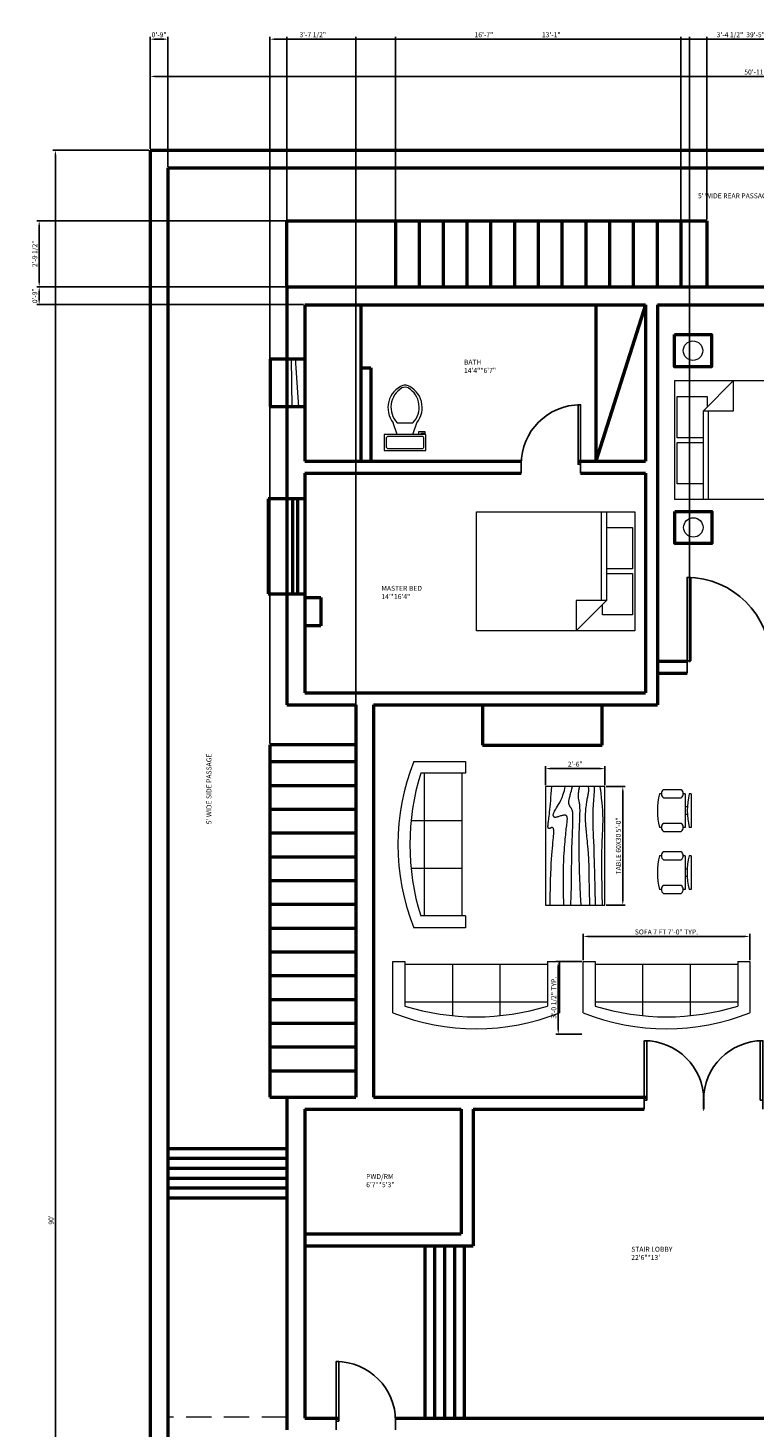
# Model space of a CAD drawing. Units: inches. Extents: x 5312 to 23584, y 2846 to 7447.
# Tile 10 of 12: x 11386 to 11753, y 3367 to 4074. Entities that reach past the tile are written whole.
import ezdxf

# ---------------------------------------------------------------- set-up
doc = ezdxf.new("R2010")
doc.units = ezdxf.units.IN
doc.linetypes.add('DASHED', pattern=[19.05, 12.7, -6.35])
for name, color, linetype, lineweight in [('A-ANNO-DIMS', 2, 'Continuous', 18), ('A-ANNO-TEXT', 3, 'Continuous', 18), ('A-AREA-IDEN', 7, 'Continuous', 18), ('A-DOOR', 4, 'Continuous', 25), ('A-FLOR-FIXT', 9, 'Continuous', 18), ('A-FLOR-OVHD', 8, 'DASHED', 18), ('A-FURN', 8, 'Continuous', 18), ('A-WALL', 7, 'Continuous', 50)]:
    doc.layers.add(name, color=color, linetype=linetype, lineweight=lineweight)
doc.styles.get("Standard").update_dxf_attribs({"font": 'arial.ttf'})
doc.dimstyles.new('ISO-25', dxfattribs={"dimtxt": 2.5, "dimasz": 2.5, "dimexe": 1.25, "dimexo": 0.625, "dimtad": 1, "dimlunit": 3, "dimtxsty": 'Standard', "dimcen": 2.5, "dimadec": 0, "dimazin": 0, "dimtfac": 1, "dimtmove": 0, "dimatfit": 3, "dimfxl": 1, "dimarcsym": 0})

# ---------------------------------------------------------------- blocks, each defined once
blk = doc.blocks.new('*U2')
for p, q in [((0, 0), (0, -6)), ((40, 0), (40, -6))]:
    blk.add_line(p, q)
blk.add_lwpolyline([(0, 0), (0, 40), (1.75, 40), (1.75, 0)], close=True)
blk.add_arc((0, 0), 40, 0, 90)
blk = doc.blocks.new('Toilet - top')
for p, q in [((9.5, -6), (9.5, -2)), ((-10, -8.5), (-8, -8.5)), ((-10, -9.5), (-10, -8.5)), ((-7, -9.5), (-10, -9.5)), ((-8, -8.5), (-8, -8)), ((-7, -8), (-7, -9.5)), ((-4, -8), (-6, -14)), ((4, -14), (-4, -14)), ((4, -8), (6, -14))]:
    blk.add_line(p, q)
blk.add_lwpolyline([(10.5, -8), (10.5, 0), (-10.5, 0), (-10.5, -8)], close=True)
for points in [[(-9.5, -2), (-9.5, -6)], [(8.5, -1), (-8.5, -1)], [(-8.5, -7), (8.5, -7)]]:
    blk.add_lwpolyline(points)
for centre, radius, start, end in [((-8.62, -1.88), 0.884, 81.8699, 188.1301), ((-8.62, -6.12), 0.884, 171.8699, 278.1301), ((8.62, -1.88), 0.884, 351.8699, 98.1301), ((8.62, -6.12), 0.884, 261.8699, 8.1301), ((3.52, -21.58), 12.17, 141.46911, 247.97143), ((4.2, -21.82), 11.33, 136.36773, 238.94682), ((-3.52, -21.58), 12.17, 292.02843, 38.53071), ((-4.2, -21.82), 11.33, 301.05301, 43.63209), ((0, -27.88), 4, 245.73182, 294.26817), ((0, -29), 4, 254.86053, 285.13947)]:
    blk.add_arc(centre, radius, start, end)
blk = doc.blocks.new('Bed - Queen')
for p, q in [((0, -80.00003), (0, 0)), ((0, 0), (59.99999, 0)), ((59.99999, 0), (59.99999, -80.00003)), ((7.99999, -1.2), (28.79998, -1.2)), ((7.99999, -14.4), (7.99999, -1.2)), ((28.79998, -1.2), (28.79998, -14.4)), ((31.19999, -1.2), (51.99999, -1.2)), ((31.19999, -14.4), (31.19999, -1.2)), ((51.99999, -1.2), (51.99999, -16.4)), ((0, -14.4), (44.8, -14.4)), ((44.8, -16.8), (0, -16.8)), ((59.99999, -29.6), (44.8, -14.4)), ((44.8, -14.4), (44.8, -29.6)), ((51.99999, -16.4), (46.79936, -16.4)), ((44.8, -29.6), (59.99999, -29.6)), ((59.99999, -80.00003), (0, -80.00003))]:
    blk.add_line(p, q)
blk = doc.blocks.new('Sofa - Roundback 7 ft.')
for p, q in [((-12.00002, -32.4421), (-12.00003, -6.5971)), ((11.99997, -32.4421), (11.99998, -6.5971)), ((-36.000027, -34), (-36.000027, -11.4696)), ((-35.999844, -13.3819), (35.9998, -13.3819)), ((35.99998, -34), (35.99998, -11.4696)), ((-36.000027, -32.4421), (35.99998, -32.4421))]:
    blk.add_line(p, q)
for points in [[(-36.000027, -34), (-42.000027, -34), (-42.000027, -8)], [(41.99998, -8), (41.99998, -34), (35.99998, -34)]]:
    blk.add_lwpolyline(points)
for centre, radius, start, end in [((0, -114.25), 114.25, 68.43141, 111.5686), ((-0.00001, -127.1968), 121.1968, 72.72033, 107.2797)]:
    blk.add_arc(centre, radius, start, end)
blk = doc.blocks.new('Table - Rectangular Woodgrain 60 x 30 in.')
for p, q in [((0, 0), (0, -30)), ((60, 0), (0, 0)), ((60, -30), (60, 0)), ((0, -30), (60, -30))]:
    blk.add_line(p, q)
for points in [[(0, -2.4), (4.8155, -2.418), (9.0302, -2.4688), (12.709, -2.5477), (15.9167, -2.65), (18.7181, -2.7711), (21.1781, -2.9063), (23.3616, -3.0508), (25.3333, -3.2), (27.1477, -3.3495), (28.8172, -3.4958), (30.3437, -3.636), (31.7291, -3.7667), (32.9756, -3.8849), (34.0849, -3.9875), (35.059, -4.0714), (35.9, -4.1334), (36.6114, -4.1711), (37.2041, -4.1854), (37.6906, -4.1779), (38.0833, -4.15), (38.3948, -4.1034), (38.6375, -4.0396), (38.8239, -3.9602), (38.9666, -3.8667), (39.0764, -3.7608), (39.1573, -3.6448), (39.2116, -3.521), (39.2416, -3.3917), (39.2498, -3.2593), (39.2385, -3.1261), (39.21, -2.9944), (39.1666, -2.8667), (39.111, -2.7447), (39.0468, -2.6281), (38.978, -2.5163), (38.9083, -2.4083), (38.8418, -2.3035), (38.7823, -2.201), (38.7337, -2.1001), (38.7, -2), (38.6844, -1.9003), (38.6875, -1.8021), (38.7094, -1.707), (38.75, -1.6167), (38.8094, -1.5326), (38.8875, -1.4563), (38.9844, -1.3893), (39.1, -1.3333), (39.2351, -1.2896), (39.3937, -1.2583), (39.5804, -1.2396), (39.8, -1.2333), (40.057, -1.2396), (40.3562, -1.2583), (40.7023, -1.2896), (41.1, -1.3333), (41.5547, -1.3895), (42.0755, -1.4573), (42.6721, -1.5361), (43.3542, -1.625), (44.1316, -1.7233), (45.014, -1.8302), (46.0114, -1.9449), (47.1333, -2.0667), (48.3862, -2.1947), (49.7625, -2.3281), (51.2513, -2.4663), (52.8416, -2.6083), (54.5226, -2.7535), (56.2833, -2.9011), (58.1127, -3.0501), (60, -3.2)], [(0, -9.2), (6.5759, -9.0858), (11.9385, -9.0365), (16.2527, -9.0418), (19.6833, -9.0917), (22.3952, -9.1759), (24.5531, -9.2844), (26.322, -9.4069), (27.8666, -9.5333), (29.3241, -9.6553), (30.7203, -9.7719), (32.0532, -9.8837), (33.3208, -9.9917), (34.5213, -10.0965), (35.6526, -10.199), (36.7128, -10.2999), (37.7, -10.4), (38.6129, -10.4996), (39.4531, -10.5969), (40.223, -10.6895), (40.925, -10.775), (41.5613, -10.8512), (42.1344, -10.9156), (42.6465, -10.966), (43.1, -11), (43.4976, -11.0158), (43.8437, -11.0136), (44.143, -10.9942), (44.4, -10.9583), (44.6195, -10.9069), (44.8062, -10.8406), (44.9648, -10.7603), (45.1, -10.6667), (45.2155, -10.5598), (45.3114, -10.4365), (45.3871, -10.2929), (45.4416, -10.125), (45.4743, -9.929), (45.4844, -9.7011), (45.4709, -9.4371), (45.4333, -9.1333), (45.3716, -8.7883), (45.2896, -8.4104), (45.1919, -8.0107), (45.0833, -7.6), (44.9685, -7.1893), (44.8521, -6.7896), (44.7388, -6.4117), (44.6333, -6.0667), (44.54, -5.7628), (44.4614, -5.4979), (44.4001, -5.2675), (44.3583, -5.0667), (44.3384, -4.8909), (44.3427, -4.7354), (44.3736, -4.5956), (44.4333, -4.4667), (44.5236, -4.3453), (44.6427, -4.2333), (44.7884, -4.1339), (44.9583, -4.05), (45.1501, -3.9849), (45.3614, -3.9417), (45.59, -3.9234), (45.8333, -3.9333), (46.0915, -3.9749), (46.3734, -4.0531), (46.6906, -4.1736), (47.0542, -4.3417), (47.4756, -4.5629), (47.9661, -4.8427), (48.5372, -5.1866), (49.2, -5.6), (49.9676, -6.0844), (50.8594, -6.625), (51.8965, -7.2031), (53.1, -7.8), (54.491, -8.3969), (56.0906, -8.975), (57.9199, -9.5156), (60, -10)], [(0, -12.8), (5.1847, -12.9322), (9.6213, -13.0323), (13.3963, -13.1059), (16.5958, -13.1583), (19.3063, -13.1952), (21.614, -13.2219), (23.6054, -13.2439), (25.3666, -13.2667), (26.9728, -13.2947), (28.4531, -13.3281), (29.8256, -13.3663), (31.1083, -13.4083), (32.3191, -13.4535), (33.476, -13.501), (34.597, -13.5501), (35.7, -13.6), (36.7984, -13.6497), (37.8875, -13.6979), (38.9578, -13.743), (40, -13.7833), (41.0047, -13.8174), (41.9625, -13.8438), (42.864, -13.8607), (43.7, -13.8667), (44.4631, -13.8604), (45.1552, -13.8417), (45.7801, -13.8104), (46.3416, -13.7667), (46.8439, -13.7104), (47.2906, -13.6417), (47.6858, -13.5604), (48.0333, -13.4667), (48.3375, -13.3608), (48.6042, -13.2448), (48.8396, -13.121), (49.05, -12.9917), (49.2417, -12.8593), (49.4208, -12.7261), (49.5937, -12.5944), (49.7667, -12.4667), (49.9452, -12.3451), (50.1323, -12.2313), (50.3303, -12.1268), (50.5416, -12.0333), (50.7686, -11.9524), (51.0135, -11.8854), (51.2788, -11.8341), (51.5666, -11.8), (51.8785, -11.7843), (52.2116, -11.7865), (52.562, -11.8059), (52.926, -11.8417), (53.2998, -11.8931), (53.6795, -11.9594), (54.0614, -12.0397), (54.4416, -12.1333), (54.8223, -12.2401), (55.2293, -12.3625), (55.6942, -12.5037), (56.2489, -12.6667), (56.9251, -12.8547), (57.7545, -13.0708), (58.7689, -13.3182), (60, -13.6)], [(0, -18), (5.124, -17.7273), (9.6609, -17.5057), (13.6705, -17.3303), (17.2125, -17.1958), (20.3467, -17.0973), (23.1328, -17.0297), (25.6307, -16.9878), (27.9, -16.9667), (29.9928, -16.9617), (31.9302, -16.9703), (33.7254, -16.9907), (35.3917, -17.0208), (36.9423, -17.0588), (38.3906, -17.1026), (39.7499, -17.1503), (41.0333, -17.2), (42.2519, -17.2496), (43.4073, -17.2969), (44.4986, -17.3395), (45.525, -17.375), (46.4858, -17.4012), (47.3802, -17.4156), (48.2074, -17.416), (48.9667, -17.4), (49.6583, -17.3662), (50.2872, -17.3167), (50.8595, -17.2547), (51.3812, -17.1833), (51.8584, -17.1057), (52.2971, -17.025), (52.7034, -16.9443), (53.0833, -16.8667), (53.443, -16.7951), (53.789, -16.7313), (54.128, -16.6768), (54.4666, -16.6334), (54.8115, -16.6024), (55.1693, -16.5854), (55.5465, -16.5841), (55.95, -16.6), (56.3828, -16.6337), (56.8346, -16.6823), (57.2915, -16.7418), (57.7396, -16.8084), (58.165, -16.878), (58.5539, -16.9469), (58.8924, -17.0111), (59.1666, -17.0667), (59.3679, -17.1107), (59.5078, -17.1438), (59.6032, -17.1675), (59.6708, -17.1833), (59.7275, -17.193), (59.7901, -17.1979), (59.8753, -17.1998), (60, -17.2)], [(0, -22.4), (8.0098, -22.2501), (14.4094, -22.1011), (19.4168, -21.9535), (23.25, -21.8083), (26.1269, -21.6663), (28.2656, -21.5281), (29.884, -21.3947), (31.2, -21.2667), (32.3967, -21.1448), (33.5172, -21.0292), (34.5697, -20.9198), (35.5625, -20.8167), (36.5037, -20.7198), (37.4015, -20.6292), (38.2642, -20.5448), (39.1, -20.4667), (39.9164, -20.3951), (40.7187, -20.3313), (41.5117, -20.2768), (42.3, -20.2333), (43.0883, -20.2024), (43.8812, -20.1854), (44.6836, -20.1841), (45.5, -20.2), (46.3328, -20.234), (47.1747, -20.2844), (48.0163, -20.3488), (48.8479, -20.425), (49.66, -20.5106), (50.4429, -20.6031), (51.1872, -20.7004), (51.8833, -20.8), (52.5246, -20.8999), (53.1166, -20.9995), (53.6681, -21.0983), (54.1875, -21.1958), (54.6834, -21.2919), (55.1646, -21.3859), (55.6394, -21.4777), (56.1167, -21.5667), (56.6028, -21.6515), (57.0961, -21.7266), (57.5929, -21.7852), (58.0896, -21.8208), (58.5823, -21.8268), (59.0674, -21.7964), (59.5412, -21.723), (60, -21.6)], [(0, -25.2), (8.6355, -25.0504), (15.7026, -24.9031), (21.4049, -24.7606), (25.9458, -24.625), (29.529, -24.4988), (32.3578, -24.3844), (34.6359, -24.284), (36.5667, -24.2), (38.3213, -24.1341), (39.9417, -24.0854), (41.437, -24.0523), (42.8167, -24.0333), (44.0901, -24.0268), (45.2667, -24.0313), (46.3557, -24.0451), (47.3667, -24.0667), (48.309, -24.0947), (49.1928, -24.1287), (50.0284, -24.168), (50.826, -24.2125), (51.5959, -24.2617), (52.3483, -24.3151), (53.0935, -24.3725), (53.8417, -24.4334), (54.6009, -24.497), (55.3699, -24.561), (56.1454, -24.6226), (56.9239, -24.6792), (57.7021, -24.7279), (58.4764, -24.7662), (59.2435, -24.7911), (60, -24.8)], [(0, -28.8), (5.6867, -28.6681), (10.45, -28.5698), (14.407, -28.5012), (17.675, -28.4584), (20.3711, -28.4374), (22.6125, -28.4344), (24.5164, -28.4455), (26.2, -28.4667), (27.762, -28.4947), (29.2276, -28.5281), (30.6033, -28.5663), (31.8958, -28.6084), (33.1118, -28.6535), (34.2578, -28.7011), (35.3405, -28.7501), (36.3666, -28.8), (37.3443, -28.8497), (38.288, -28.8974), (39.2137, -28.9412), (40.1375, -28.9792), (41.0753, -29.0093), (42.0432, -29.0297), (43.0572, -29.0384), (44.1333, -29.0333), (45.2936, -29.0114), (46.5843, -28.9641), (48.0579, -28.8816), (49.7666, -28.7542), (51.7629, -28.5721), (54.0989, -28.3255), (56.8272, -28.0048), (60, -27.6)]]:
    blk.add_lwpolyline(points)
blk = doc.blocks.new('Chair - Desk')
for p, q in [((-8.5, 0), (-8.5, -1)), ((-8.5, 0), (8.5, 0)), ((8.5, 0), (8.5, -1)), ((-10.5, -5), (-10.5, -14)), ((-8.5, -3), (-8.5, -4)), ((-8.5, -3), (8.5, -3)), ((-6.5, -14), (-6.5, -5)), ((-2, -3), (-2, -1.9355)), ((2, -1.9576), (2, -3)), ((6.5, -5), (6.5, -14)), ((8.5, -3), (8.5, -4)), ((10.5, -14), (10.5, -5)), ((-8.5, -15), (-8.5, -16)), ((8.5, -15), (8.5, -16))]:
    blk.add_line(p, q)
for centre, radius, start, end in [((-8.5, -6.5), 2.5, 36.8699, 143.1301), ((0, 34.625), 36.625, 256.5803, 283.4197), ((8.5, -6.5), 2.5, 36.8699, 143.1301), ((-8.5, -12.5), 2.5, 216.8699, 323.1301), ((8.5, -12.5), 2.5, 216.8699, 323.1301), ((0, 19.625), 36.625, 256.5803, 283.4197)]:
    blk.add_arc(centre, radius, start, end)
blk = doc.blocks.new('*D19')
at = {"layer": 'A-ANNO-DIMS', "color": 0, "lineweight": -2, "transparency": 16777216}
for p, q in [((11447.29, 4012.53), (11447.29, 4050.35)), ((11449.79, 4049.1), (12055.79, 4049.1)), ((12058.29, 4012.53), (12058.29, 4050.35))]:
    blk.add_line(p, q, dxfattribs=at)
at = {"layer": 'A-ANNO-DIMS', "color": 0, "transparency": 16777216}
for points in [[(11449.79, 4049.52), (11449.79, 4048.69), (11447.29, 4049.1)], [(12055.79, 4049.52), (12055.79, 4048.69), (12058.29, 4049.1)]]:
    blk.add_solid(points, dxfattribs=at)
at = {"layer": 'DEFPOINTS', "color": 0, "transparency": 16777216}
for p in [(12058.29, 4049.1), (11447.29, 4011.91), (12058.29, 4011.91)]:
    blk.add_point(p, dxfattribs=at)
at = {"layer": 'A-ANNO-DIMS', "color": 0, "transparency": 16777216, "insert": (11752.79, 4051.01), "char_height": 2.5, "attachment_point": 5}
blk.add_mtext('50\'-11"', dxfattribs=at)
blk = doc.blocks.new('*D20')
at = {"layer": 'A-ANNO-DIMS', "color": 0, "lineweight": -2, "transparency": 16777216}
for p, q in [((11446.67, 4011.91), (11398.24, 4011.91)), ((11399.49, 4009.41), (11399.49, 2934.41)), ((11446.67, 2931.91), (11398.24, 2931.91))]:
    blk.add_line(p, q, dxfattribs=at)
at = {"layer": 'A-ANNO-DIMS', "color": 0, "transparency": 16777216}
for points in [[(11399.07, 4009.41), (11399.9, 4009.41), (11399.49, 4011.91)], [(11399.07, 2934.41), (11399.9, 2934.41), (11399.49, 2931.91)]]:
    blk.add_solid(points, dxfattribs=at)
at = {"layer": 'DEFPOINTS', "color": 0, "transparency": 16777216}
for p in [(11447.29, 4011.91), (11399.49, 2931.91), (11447.29, 2931.91)]:
    blk.add_point(p, dxfattribs=at)
at = {"layer": 'A-ANNO-DIMS', "color": 0, "transparency": 16777216, "insert": (11397.59, 3471.91), "char_height": 2.5, "attachment_point": 5, "rotation": 90}
blk.add_mtext("90'", dxfattribs=at)
blk = doc.blocks.new('WARDROBE-HANGER')
for p, q in [((0, 3.4), (24.8, 3.4)), ((0, 1.32), (24.99, 0))]:
    blk.add_line(p, q)
blk = doc.blocks.new('*D27')
at = {"layer": 'A-ANNO-DIMS', "color": 0, "lineweight": -2, "transparency": 16777216}
for p, q in [((11665.83, 3603.06), (11665.83, 3616.28)), ((11747.33, 3615.03), (11668.33, 3615.03)), ((11749.83, 3603.06), (11749.83, 3616.28))]:
    blk.add_line(p, q, dxfattribs=at)
at = {"layer": 'A-ANNO-DIMS', "color": 0, "transparency": 16777216}
for points in [[(11668.33, 3615.45), (11668.33, 3614.62), (11665.83, 3615.03)], [(11747.33, 3615.45), (11747.33, 3614.62), (11749.83, 3615.03)]]:
    blk.add_solid(points, dxfattribs=at)
at = {"layer": 'DEFPOINTS', "color": 0, "transparency": 16777216}
for p in [(11665.83, 3615.03), (11665.83, 3602.43), (11749.83, 3602.43)]:
    blk.add_point(p, dxfattribs=at)
at = {"layer": 'A-ANNO-DIMS', "color": 0, "transparency": 16777216, "insert": (11707.83, 3616.95), "char_height": 2.5, "attachment_point": 5, "rotation": 359.99998}
blk.add_mtext('SOFA 7 FT 7\'-0" TYP.', dxfattribs=at)
blk = doc.blocks.new('*D28')
at = {"layer": 'A-ANNO-DIMS', "color": 0, "lineweight": -2, "transparency": 16777216}
for p, q in [((11665.21, 3602.43), (11651.98, 3602.43)), ((11653.23, 3599.93), (11653.23, 3568.27)), ((11665.21, 3565.77), (11651.98, 3565.77))]:
    blk.add_line(p, q, dxfattribs=at)
at = {"layer": 'A-ANNO-DIMS', "color": 0, "transparency": 16777216}
for points in [[(11652.81, 3599.93), (11653.65, 3599.93), (11653.23, 3602.43)], [(11652.81, 3568.27), (11653.65, 3568.27), (11653.23, 3565.77)]]:
    blk.add_solid(points, dxfattribs=at)
at = {"layer": 'DEFPOINTS', "color": 0, "transparency": 16777216}
for p in [(11665.83, 3602.43), (11653.23, 3565.77), (11665.83, 3565.77)]:
    blk.add_point(p, dxfattribs=at)
at = {"layer": 'A-ANNO-DIMS', "color": 0, "transparency": 16777216, "insert": (11651.31, 3584.1), "char_height": 2.5, "attachment_point": 5, "rotation": 90}
blk.add_mtext('3\'-0 1/2" TYP.', dxfattribs=at)
blk = doc.blocks.new('*D41')
at = {"layer": 'A-ANNO-DIMS', "color": 0, "lineweight": -2, "transparency": 16777216}
for p, q in [((11677.43, 3690.74), (11687.05, 3690.74)), ((11685.8, 3633.24), (11685.8, 3688.24)), ((11677.43, 3630.74), (11687.05, 3630.74))]:
    blk.add_line(p, q, dxfattribs=at)
at = {"layer": 'A-ANNO-DIMS', "color": 0, "transparency": 16777216}
for points in [[(11685.39, 3688.24), (11686.22, 3688.24), (11685.8, 3690.74)], [(11685.39, 3633.24), (11686.22, 3633.24), (11685.8, 3630.74)]]:
    blk.add_solid(points, dxfattribs=at)
at = {"layer": 'DEFPOINTS', "color": 0, "transparency": 16777216}
for p in [(11676.8, 3690.74), (11685.8, 3690.74), (11676.8, 3630.74)]:
    blk.add_point(p, dxfattribs=at)
at = {"layer": 'A-ANNO-DIMS', "color": 0, "transparency": 16777216, "insert": (11683.9, 3660.74), "char_height": 2.5, "attachment_point": 5, "rotation": 90}
blk.add_mtext('TABLE 60X30 5\'-0"', dxfattribs=at)
blk = doc.blocks.new('*D42')
at = {"layer": 'A-ANNO-DIMS', "color": 0, "lineweight": -2, "transparency": 16777216}
for p, q in [((11646.8, 3691.36), (11646.8, 3700.99)), ((11674.3, 3699.74), (11649.3, 3699.74)), ((11676.8, 3691.36), (11676.8, 3700.99))]:
    blk.add_line(p, q, dxfattribs=at)
at = {"layer": 'A-ANNO-DIMS', "color": 0, "transparency": 16777216}
for points in [[(11649.3, 3700.15), (11649.3, 3699.32), (11646.8, 3699.74)], [(11674.3, 3700.15), (11674.3, 3699.32), (11676.8, 3699.74)]]:
    blk.add_solid(points, dxfattribs=at)
at = {"layer": 'DEFPOINTS', "color": 0, "transparency": 16777216}
for p in [(11646.8, 3699.74), (11646.8, 3690.74), (11676.8, 3690.74)]:
    blk.add_point(p, dxfattribs=at)
at = {"layer": 'A-ANNO-DIMS', "color": 0, "transparency": 16777216, "insert": (11661.8, 3701.64), "char_height": 2.5, "attachment_point": 5}
blk.add_mtext('2\'-6"', dxfattribs=at)
blk = doc.blocks.new('*D59')
at = {"layer": 'A-ANNO-DIMS', "color": 0, "lineweight": -2, "transparency": 16777216}
for p, q in [((11516.29, 3943.53), (11516.29, 4069.16)), ((11518.79, 4067.91), (11986.79, 4067.91)), ((11989.29, 3943.53), (11989.29, 4069.16))]:
    blk.add_line(p, q, dxfattribs=at)
at = {"layer": 'A-ANNO-DIMS', "color": 0, "transparency": 16777216}
for points in [[(11518.79, 4068.32), (11518.79, 4067.49), (11516.29, 4067.91)], [(11986.79, 4068.32), (11986.79, 4067.49), (11989.29, 4067.91)]]:
    blk.add_solid(points, dxfattribs=at)
at = {"layer": 'DEFPOINTS', "color": 0, "transparency": 16777216}
for p in [(11989.29, 4067.91), (11516.29, 3942.91), (11989.29, 3942.91)]:
    blk.add_point(p, dxfattribs=at)
at = {"layer": 'A-ANNO-DIMS', "color": 0, "transparency": 16777216, "insert": (11752.79, 4069.81), "char_height": 2.5, "attachment_point": 5}
blk.add_mtext('39\'-5"', dxfattribs=at)
blk = doc.blocks.new('*D61')
at = {"layer": 'A-ANNO-DIMS', "color": 0, "lineweight": -2, "transparency": 16777216}
for p, q in [((11516.29, 3943.53), (11516.29, 4069.16)), ((11518.79, 4067.91), (11712.61, 4067.91)), ((11715.11, 3943.53), (11715.11, 4069.16))]:
    blk.add_line(p, q, dxfattribs=at)
at = {"layer": 'A-ANNO-DIMS', "color": 0, "transparency": 16777216}
for points in [[(11518.79, 4068.32), (11518.79, 4067.49), (11516.29, 4067.91)], [(11712.61, 4068.32), (11712.61, 4067.49), (11715.11, 4067.91)]]:
    blk.add_solid(points, dxfattribs=at)
at = {"layer": 'DEFPOINTS', "color": 0, "transparency": 16777216}
for p in [(11715.11, 4067.91), (11516.29, 3942.91), (11715.11, 3942.91)]:
    blk.add_point(p, dxfattribs=at)
at = {"layer": 'A-ANNO-DIMS', "color": 0, "transparency": 16777216, "insert": (11615.7, 4069.81), "char_height": 2.5, "attachment_point": 5}
blk.add_mtext('16\'-7"', dxfattribs=at)
blk = doc.blocks.new('*D65')
at = {"layer": 'A-ANNO-DIMS', "color": 0, "lineweight": -2, "transparency": 16777216}
for p, q in [((11447.29, 4012.53), (11447.29, 4069.16)), ((11449.79, 4067.91), (11453.79, 4067.91)), ((11456.29, 4003.53), (11456.29, 4069.16))]:
    blk.add_line(p, q, dxfattribs=at)
at = {"layer": 'A-ANNO-DIMS', "color": 0, "transparency": 16777216}
for points in [[(11449.79, 4068.32), (11449.79, 4067.49), (11447.29, 4067.91)], [(11453.79, 4068.32), (11453.79, 4067.49), (11456.29, 4067.91)]]:
    blk.add_solid(points, dxfattribs=at)
at = {"layer": 'DEFPOINTS', "color": 0, "transparency": 16777216}
for p in [(11456.29, 4067.91), (11447.29, 4011.91), (11456.29, 4002.91)]:
    blk.add_point(p, dxfattribs=at)
at = {"layer": 'A-ANNO-DIMS', "color": 0, "transparency": 16777216, "insert": (11451.79, 4069.81), "char_height": 2.5, "attachment_point": 5}
blk.add_mtext('0\'-9"', dxfattribs=at)
blk = doc.blocks.new('*D66')
at = {"layer": 'A-ANNO-DIMS', "color": 0, "lineweight": -2, "transparency": 16777216}
for p, q in [((11515.67, 3942.91), (11390.04, 3942.91)), ((11391.29, 3940.41), (11391.29, 3936.41)), ((11524.67, 3933.91), (11390.04, 3933.91))]:
    blk.add_line(p, q, dxfattribs=at)
at = {"layer": 'A-ANNO-DIMS', "color": 0, "transparency": 16777216}
for points in [[(11390.87, 3940.41), (11391.71, 3940.41), (11391.29, 3942.91)], [(11390.87, 3936.41), (11391.71, 3936.41), (11391.29, 3933.91)]]:
    blk.add_solid(points, dxfattribs=at)
at = {"layer": 'DEFPOINTS', "color": 0, "transparency": 16777216}
for p in [(11516.29, 3942.91), (11391.29, 3933.91), (11525.29, 3933.91)]:
    blk.add_point(p, dxfattribs=at)
at = {"layer": 'A-ANNO-DIMS', "color": 0, "transparency": 16777216, "insert": (11389.39, 3938.41), "char_height": 2.5, "attachment_point": 5, "rotation": 90}
blk.add_mtext('0\'-9"', dxfattribs=at)
blk = doc.blocks.new('*D67')
at = {"layer": 'A-ANNO-DIMS', "color": 0, "lineweight": -2, "transparency": 16777216}
for p, q in [((11507.65, 3712.39), (11507.65, 4069.16)), ((11510.15, 4067.91), (11548.53, 4067.91)), ((11551.03, 3712.39), (11551.03, 4069.16))]:
    blk.add_line(p, q, dxfattribs=at)
at = {"layer": 'A-ANNO-DIMS', "color": 0, "transparency": 16777216}
for points in [[(11510.15, 4068.32), (11510.15, 4067.49), (11507.65, 4067.91)], [(11548.53, 4068.32), (11548.53, 4067.49), (11551.03, 4067.91)]]:
    blk.add_solid(points, dxfattribs=at)
at = {"layer": 'DEFPOINTS', "color": 0, "transparency": 16777216}
for p in [(11551.03, 4067.91), (11507.65, 3711.77), (11551.03, 3711.77)]:
    blk.add_point(p, dxfattribs=at)
at = {"layer": 'A-ANNO-DIMS', "color": 0, "transparency": 16777216, "insert": (11529.34, 4069.83), "char_height": 2.5, "attachment_point": 5}
blk.add_mtext('3\'-7 1/2"', dxfattribs=at)
blk = doc.blocks.new('*D68')
at = {"layer": 'A-ANNO-DIMS', "color": 0, "lineweight": -2, "transparency": 16777216}
for p, q in [((11571.11, 3976.83), (11571.11, 4069.16)), ((11573.61, 4067.91), (11725.77, 4067.91)), ((11728.27, 3976.83), (11728.27, 4069.16))]:
    blk.add_line(p, q, dxfattribs=at)
at = {"layer": 'A-ANNO-DIMS', "color": 0, "transparency": 16777216}
for points in [[(11573.61, 4068.32), (11573.61, 4067.49), (11571.11, 4067.91)], [(11725.77, 4068.32), (11725.77, 4067.49), (11728.27, 4067.91)]]:
    blk.add_solid(points, dxfattribs=at)
at = {"layer": 'DEFPOINTS', "color": 0, "transparency": 16777216}
for p in [(11728.27, 4067.91), (11571.11, 3976.21), (11728.27, 3976.21)]:
    blk.add_point(p, dxfattribs=at)
at = {"layer": 'A-ANNO-DIMS', "color": 0, "transparency": 16777216, "insert": (11649.69, 4069.81), "char_height": 2.5, "attachment_point": 5}
blk.add_mtext('13\'-1"', dxfattribs=at)
blk = doc.blocks.new('*D69')
at = {"layer": 'A-ANNO-DIMS', "color": 0, "lineweight": -2, "transparency": 16777216}
for p, q in [((11570.48, 3976.21), (11390.04, 3976.21)), ((11391.29, 3973.71), (11391.29, 3945.41)), ((11570.48, 3942.91), (11390.04, 3942.91))]:
    blk.add_line(p, q, dxfattribs=at)
at = {"layer": 'A-ANNO-DIMS', "color": 0, "transparency": 16777216}
for points in [[(11390.87, 3973.71), (11391.71, 3973.71), (11391.29, 3976.21)], [(11390.87, 3945.41), (11391.71, 3945.41), (11391.29, 3942.91)]]:
    blk.add_solid(points, dxfattribs=at)
at = {"layer": 'DEFPOINTS', "color": 0, "transparency": 16777216}
for p in [(11571.11, 3976.21), (11391.29, 3942.91), (11571.11, 3942.91)]:
    blk.add_point(p, dxfattribs=at)
at = {"layer": 'A-ANNO-DIMS', "color": 0, "transparency": 16777216, "insert": (11389.37, 3959.56), "char_height": 2.5, "attachment_point": 5, "rotation": 90}
blk.add_mtext('2\'-9 1/2"', dxfattribs=at)
blk = doc.blocks.new('*D70')
at = {"layer": 'A-ANNO-DIMS', "color": 0, "lineweight": -2, "transparency": 16777216}
for p, q in [((11719.53, 3753.53), (11719.53, 4069.16)), ((11722.03, 4067.91), (11757.73, 4067.91)), ((11760.23, 3752.99), (11760.23, 4069.16))]:
    blk.add_line(p, q, dxfattribs=at)
at = {"layer": 'A-ANNO-DIMS', "color": 0, "transparency": 16777216}
for points in [[(11722.03, 4068.32), (11722.03, 4067.49), (11719.53, 4067.91)], [(11757.73, 4068.32), (11757.73, 4067.49), (11760.23, 4067.91)]]:
    blk.add_solid(points, dxfattribs=at)
at = {"layer": 'DEFPOINTS', "color": 0, "transparency": 16777216}
for p in [(11760.23, 4067.91), (11719.53, 3752.91), (11760.23, 3752.37)]:
    blk.add_point(p, dxfattribs=at)
at = {"layer": 'A-ANNO-DIMS', "color": 0, "transparency": 16777216, "insert": (11739.88, 4069.83), "char_height": 2.5, "attachment_point": 5}
blk.add_mtext('3\'-4 1/2"', dxfattribs=at)

msp = doc.modelspace()

# ---------------------------------------------------------------- linework, layer by layer
at = {"layer": 'A-FLOR-OVHD'}
msp.add_line((11516.292, 3372.371), (11456.292, 3372.371), dxfattribs=at)
at = {"layer": 'A-FURN'}
for centre in [(11721.219, 3910.691), (11721.401, 3821.458)]:
    msp.add_circle(centre, 4.897, dxfattribs=at)
at = {"layer": 'A-WALL'}
for p, q in [((11447.292, 4011.907), (12058.292, 4011.907)), ((11447.292, 4011.907), (11447.292, 2931.907)), ((11456.292, 4002.907), (11456.292, 2940.907)), ((11456.292, 4002.907), (12049.292, 4002.907)), ((11516.292, 3942.907), (11516.292, 3976.209)), ((11516.292, 3976.209), (11728.274, 3976.209)), ((11571.108, 3976.209), (11571.108, 3942.907)), ((11583.108, 3976.209), (11583.108, 3942.907)), ((11595.108, 3976.209), (11595.108, 3942.907)), ((11607.108, 3976.209), (11607.108, 3942.907)), ((11619.108, 3976.209), (11619.108, 3942.907)), ((11631.108, 3976.209), (11631.108, 3942.907)), ((11643.108, 3976.209), (11643.108, 3942.907)), ((11655.108, 3976.209), (11655.108, 3942.907)), ((11667.108, 3976.209), (11667.108, 3942.907)), ((11679.108, 3976.209), (11679.108, 3942.907)), ((11691.108, 3976.209), (11691.108, 3942.907)), ((11703.108, 3976.209), (11703.108, 3942.907)), ((11715.108, 3976.209), (11715.108, 3942.907)), ((11728.274, 3976.209), (11728.274, 3942.907)), ((11516.292, 3942.907), (11516.292, 3731.907)), ((11516.292, 3942.907), (11989.292, 3942.907)), ((11525.292, 3933.907), (11525.292, 3854.907)), ((11525.292, 3933.907), (11697.292, 3933.907)), ((11553.556, 3933.907), (11553.556, 3854.907)), ((11672.22, 3933.907), (11672.22, 3854.907)), ((11697.292, 3933.907), (11672.22, 3854.907)), ((11697.292, 3933.907), (11697.292, 3854.907)), ((11703.292, 3933.907), (11703.292, 3731.907)), ((11703.292, 3933.907), (11980.292, 3933.907)), ((11525.292, 3906.467), (11507.917, 3906.467)), ((11507.917, 3906.467), (11507.917, 3882.467)), ((11553.556, 3901.978), (11558.577, 3901.978)), ((11558.577, 3901.978), (11558.577, 3854.907)), ((11507.917, 3882.467), (11525.292, 3882.467)), ((11525.292, 3854.907), (11634.556, 3854.907)), ((11663.205, 3854.907), (11697.292, 3854.907)), ((11525.292, 3848.907), (11634.517, 3848.907)), ((11525.292, 3848.907), (11525.292, 3737.907)), ((11664.517, 3848.907), (11697.292, 3848.907)), ((11697.292, 3848.907), (11697.292, 3737.907)), ((11525.292, 3835.907), (11506.889, 3835.907)), ((11506.889, 3835.907), (11506.889, 3787.907)), ((11519.1, 3835.907), (11519.1, 3787.907)), ((11521.562, 3835.907), (11521.562, 3787.907)), ((11506.889, 3787.907), (11525.292, 3787.907)), ((11525.292, 3786.114), (11533.455, 3786.114)), ((11533.455, 3786.114), (11533.455, 3771.742)), ((11533.455, 3771.742), (11525.292, 3771.742)), ((11703.292, 3753.907), (11718.226, 3753.907)), ((11703.292, 3747.907), (11718.226, 3747.907)), ((11516.292, 3731.907), (11551.031, 3731.907)), ((11525.292, 3737.907), (11697.292, 3737.907)), ((11551.031, 3731.907), (11551.031, 3533.907)), ((11560.031, 3731.907), (11560.031, 3533.907)), ((11560.031, 3731.907), (11703.292, 3731.907)), ((11615.066, 3731.907), (11615.066, 3711.594)), ((11675.367, 3711.594), (11675.367, 3731.907)), ((11551.031, 3711.769), (11507.652, 3711.769)), ((11507.652, 3711.769), (11507.652, 3533.907)), ((11615.066, 3711.594), (11675.367, 3711.594)), ((11507.652, 3703.261), (11551.031, 3703.261)), ((11507.652, 3691.261), (11551.031, 3691.261)), ((11507.652, 3679.261), (11551.031, 3679.261)), ((11507.652, 3667.261), (11551.031, 3667.261)), ((11507.652, 3655.261), (11551.031, 3655.261)), ((11507.652, 3643.261), (11551.031, 3643.261)), ((11507.652, 3631.261), (11551.031, 3631.261)), ((11507.652, 3619.261), (11551.031, 3619.261)), ((11507.652, 3607.261), (11551.031, 3607.261)), ((11507.652, 3595.261), (11551.031, 3595.261)), ((11507.652, 3583.261), (11551.031, 3583.261)), ((11507.652, 3571.261), (11551.031, 3571.261)), ((11507.652, 3559.261), (11551.031, 3559.261)), ((11507.652, 3547.261), (11551.031, 3547.261)), ((11507.652, 3533.907), (11516.292, 3533.907)), ((11516.292, 3533.907), (11551.031, 3533.907)), ((11516.292, 3533.907), (11516.292, 3365.907)), ((11560.031, 3533.907), (11697.936, 3533.907)), ((11726.555, 3533.907), (11726.586, 3533.907)), ((11525.292, 3527.907), (11604.292, 3527.907)), ((11525.292, 3527.907), (11525.292, 3371.907)), ((11604.292, 3527.907), (11604.292, 3464.907)), ((11610.292, 3527.907), (11610.292, 3458.907)), ((11610.292, 3527.907), (11696.624, 3527.907)), ((11726.517, 3527.907), (11726.624, 3527.907)), ((11456.292, 3508.062), (11516.292, 3508.062)), ((11456.292, 3503.062), (11516.292, 3503.062)), ((11456.292, 3498.062), (11516.292, 3498.062)), ((11456.292, 3493.062), (11516.292, 3493.062)), ((11456.292, 3488.062), (11516.292, 3488.062)), ((11456.292, 3483.062), (11516.292, 3483.062)), ((11525.292, 3464.907), (11604.292, 3464.907)), ((11525.292, 3458.907), (11610.292, 3458.907)), ((11585.832, 3458.907), (11585.832, 3371.907)), ((11590.832, 3458.907), (11590.832, 3371.907)), ((11595.832, 3458.907), (11595.832, 3371.907)), ((11600.832, 3458.907), (11600.832, 3371.907)), ((11605.832, 3458.907), (11605.832, 3371.907)), ((11525.292, 3371.907), (11542.463, 3371.907)), ((11571.113, 3371.907), (11980.292, 3371.907))]:
    msp.add_line(p, q, dxfattribs=at)
for points in [[(11711.871, 3918.8), (11730.567, 3918.8), (11730.567, 3902.583), (11711.871, 3902.583)], [(11712.054, 3829.566), (11730.749, 3829.566), (11730.749, 3813.349), (11712.054, 3813.349)]]:
    msp.add_lwpolyline(points, close=True, dxfattribs=at)

# ---------------------------------------------------------------- block references
at = {"layer": 'A-DOOR'}
for p, xscale, yscale, zscale in [((11664.517, 3853.377), -0.75, 0.75, 0.75), ((11718.226, 3754.207), 1.049999999999999, 1.049999999999999, 1.049999999999999), ((11696.624, 3532.407), 0.75, 0.75, 0.75), ((11756.517, 3532.407), -0.75, 0.75, 0.75), ((11541.15, 3370.407), 0.75, 0.75, 0.75)]:
    msp.add_blockref('*U2', p, dxfattribs=dict(at, xscale=xscale, yscale=yscale, zscale=zscale))
at = {"layer": 'A-FLOR-FIXT', "rotation": 180}
msp.add_blockref('Toilet - top', (11575.923, 3860.329), dxfattribs=at)
at = {"layer": 'A-FURN'}
for name, p, rotation in [('WARDROBE-HANGER', (11517.068, 3906.742), 274.0153839270132), ('Bed - Queen', (11712.054, 3835.548), 90), ('Bed - Queen', (11691.923, 3829.357), 270), ('Sofa - Roundback 7 ft.', (11572.361, 3661.389), 90), ('Table - Rectangular Woodgrain 60 x 30 in.', (11646.802, 3630.736), 90), ('Chair - Desk', (11720.319, 3678.547), 270), ('Chair - Desk', (11720.27, 3647.227), 270), ('Sofa - Roundback 7 ft.', (11611.825, 3568.432), 179.9999778310086), ('Sofa - Roundback 7 ft.', (11707.831, 3568.432), 179.9999778310086)]:
    msp.add_blockref(name, p, dxfattribs=dict(at, rotation=rotation))

# ---------------------------------------------------------------- texts
at = {"layer": 'A-ANNO-TEXT', "insert": (11723.753, 3990.095), "char_height": 2.5, "attachment_point": 1}
msp.add_mtext_dynamic_manual_height_columns("5' WIDE REAR PASSAGE", width=78.67751, gutter_width=12.5, heights=[0], dxfattribs=at)
at = {"layer": 'A-ANNO-TEXT', "insert": (11475.715, 3671.671), "char_height": 2.5, "attachment_point": 1, "rotation": 90}
msp.add_mtext_dynamic_manual_height_columns("5' WIDE SIDE PASSAGE", width=39.96532, gutter_width=12.5, heights=[0], dxfattribs=at)
at = {"layer": 'A-AREA-IDEN', "char_height": 2.5, "attachment_point": 1}
for s, width, insert in [('BATH\\P14\'4"*6\'7"', 46.79653, (11605.652, 3906.143)), ('MASTER BED\\P14\'*16\'4"', 43.61852, (11564.006, 3791.988)), ('PWD/RM\\P6\'7"*5\'3"', 35.47189, (11556.303, 3495.091)), ('STAIR LOBBY\\P22\'6"*13\'', 91.08094, (11690.077, 3458.371))]:
    msp.add_mtext_dynamic_manual_height_columns(s, width=width, gutter_width=12.5, heights=[0], dxfattribs=dict(at, insert=insert))

# ---------------------------------------------------------------- dimensions: what is measured, and where the dimension line sits
at = {"layer": 'A-ANNO-DIMS'}
for base, p1, p2, override, picture, middle in [((11456.292, 4067.907), (11447.292, 4011.907), (11456.292, 4002.907), {"dimdec": 1, "dimlfac": 1, "dimrnd": 0, "dimzin": 1, "dimdsep": 46, "dimlunit": 4, "dimfrac": 2}, '*D65', (11451.792, 4069.809)), ((11551.031, 4067.907), (11507.652, 3711.769), (11551.031, 3711.769), {"dimdec": 1, "dimlfac": 1, "dimrnd": 0, "dimzin": 1, "dimdsep": 46, "dimlunit": 4, "dimfrac": 2}, '*D67', (11529.341, 4069.826)), ((11989.292, 4067.907), (11516.292, 3942.907), (11989.292, 3942.907), {"dimdec": 1, "dimlfac": 1, "dimrnd": 0, "dimzin": 1, "dimdsep": 46, "dimlunit": 4, "dimfrac": 2}, '*D59', (11752.792, 4069.809)), ((11715.108, 4067.907), (11516.292, 3942.907), (11715.108, 3942.907), {"dimdec": 1, "dimlfac": 1, "dimrnd": 0, "dimzin": 1, "dimdsep": 46, "dimlunit": 4, "dimfrac": 2}, '*D61', (11615.7, 4069.809)), ((11728.274, 4067.907), (11571.108, 3976.209), (11728.274, 3976.209), {"dimdec": 1, "dimlfac": 1, "dimrnd": 0, "dimzin": 1, "dimdsep": 46, "dimlunit": 4, "dimfrac": 2}, '*D68', (11649.691, 4069.809)), ((11760.226, 4067.907), (11719.526, 3752.908), (11760.226, 3752.37), {"dimdec": 1, "dimlfac": 1, "dimrnd": 0, "dimzin": 1, "dimdsep": 46, "dimlunit": 4, "dimfrac": 2}, '*D70', (11739.876, 4069.826)), ((12058.292, 4049.105), (11447.292, 4011.907), (12058.292, 4011.907), {"dimclrd": 0, "dimclre": 0, "dimclrt": 0}, '*D19', (11752.792, 4051.006))]:
    dim = msp.add_linear_dim(base=base, p1=p1, p2=p2, dimstyle='ISO-25', override=override, dxfattribs=at)
    dim.commit()
    dim.dimension.update_dxf_attribs({"geometry": picture, "text_midpoint": middle})
for base, p1, p2, angle, override, picture, middle in [((11399.487, 2931.907), (11447.292, 4011.907), (11447.292, 2931.907), 90, {"dimclrd": 0, "dimclre": 0, "dimclrt": 0}, '*D20', (11397.586, 3471.907)), ((11391.292, 3942.907), (11571.108, 3976.209), (11571.108, 3942.907), 90, {"dimdec": 1, "dimlfac": 1, "dimrnd": 0, "dimzin": 1, "dimdsep": 46, "dimlunit": 4, "dimfrac": 2}, '*D69', (11389.374, 3959.558)), ((11391.292, 3933.907), (11516.292, 3942.907), (11525.292, 3933.907), 90, {"dimdec": 1, "dimlfac": 1, "dimrnd": 0, "dimzin": 1, "dimdsep": 46, "dimlunit": 4, "dimfrac": 2}, '*D66', (11389.39, 3938.407)), ((11646.802, 3699.736), (11676.802, 3690.736), (11646.802, 3690.736), 180, {"dimdec": 1, "dimrnd": 0, "dimzin": 1, "dimlunit": 4, "dimfrac": 2}, '*D42', (11661.802, 3701.637))]:
    dim = msp.add_linear_dim(base=base, p1=p1, p2=p2, angle=angle, dimstyle='ISO-25', override=override, dxfattribs=at)
    dim.commit()
    dim.dimension.update_dxf_attribs({"geometry": picture, "text_midpoint": middle})
for base, p1, p2, angle, text, picture, middle in [((11685.802, 3690.736), (11676.802, 3630.736), (11676.802, 3690.736), 90, 'TABLE 60X30 <>', '*D41', (11683.899, 3660.736)), ((11665.831, 3615.032), (11749.831, 3602.432), (11665.831, 3602.432), 179.999978, 'SOFA 7 FT <> TYP.', '*D27', (11707.831, 3616.951)), ((11653.231, 3565.766), (11665.831, 3602.432), (11665.831, 3565.766), 269.999978, '<> TYP.', '*D28', (11651.312, 3584.099))]:
    dim = msp.add_linear_dim(base=base, p1=p1, p2=p2, angle=angle, text=text, dimstyle='ISO-25', override={"dimdec": 1, "dimrnd": 0, "dimzin": 1, "dimlunit": 4, "dimfrac": 2}, dxfattribs=at)
    dim.commit()
    dim.dimension.update_dxf_attribs({"geometry": picture, "text_midpoint": middle})

doc.saveas('drawing.dxf')
